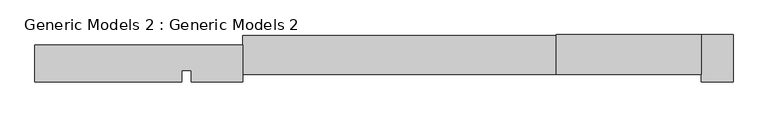
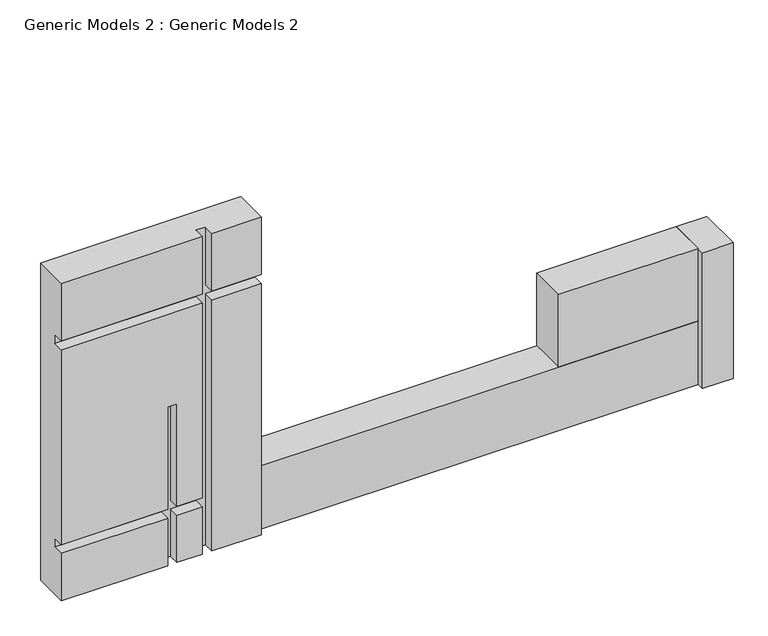
"""IFC4 building model written with IfcOpenShell, lengths in millimetres: proxy geometry, Generic Models 2 : Generic Models 2."""

from ifc_helpers import new_model, si_unit, frame, origin, place, context, project, spatial, polyline, outline, extrude, faceted_brep, source, transform, mapped, element, save


def generic_models_2_generic_models_2_1caf7409(model_context):
    return source(origin(), model_context, "Body", "SolidModel", [
        extrude(outline(polyline([(7416.0108478, -4009.874389), (7416.0108478, -3491.6545867), (9316.5582436, -3491.6545867), (9316.5582436, -4009.874389), (7416.0108478, -4009.874389)])), frame((0.0, 0.0, 4267.2), z_axis=(0.0, 0.0, 1.0), x_axis=(1.0, 0.0, 0.0)), (0.0, 0.0, 1.0), 1041.4),
        extrude(outline(polyline([(9733.554407, -4111.474389), (9316.5582436, -4111.474389), (9316.5582436, -3491.6545867), (9733.554407, -3491.6545867), (9733.554407, -4111.474389)])), frame((0.0, 0.0, 3352.8), z_axis=(0.0, 0.0, 1.0), x_axis=(1.0, 0.0, 0.0)), (0.0, 0.0, 1.0), 1955.8),
        extrude(outline(polyline([(9316.5582436, -4009.874389), (3313.273546, -4009.874389), (3313.273546, -3501.874389), (9316.5582436, -3501.874389), (9316.5582436, -4009.874389)])), frame((0.0, 0.0, 3352.8), z_axis=(0.0, 0.0, 1.0), x_axis=(1.0, 0.0, 0.0)), (0.0, 0.0, 1.0), 914.4),
        faceted_brep([(3313.273546, -4111.474389, 7924.8), (2638.6516969, -4111.474389, 7924.8), (2638.6516969, -4111.474389, 7095.4038204), (3313.273546, -4111.474389, 7095.4038204), (2511.6516969, -4111.474389, 7924.8), (589.554407, -4111.474389, 7924.8), (589.554407, -4111.474389, 7095.4038204), (2511.6516969, -4111.474389, 7095.4038204), (2638.6516969, -4111.474389, 3352.8), (3313.273546, -4111.474389, 3352.8), (3313.273546, -4111.474389, 6968.4038204), (2638.6516969, -4111.474389, 6968.4038204), (2511.6516969, -4111.474389, 6968.4038204), (589.554407, -4111.474389, 6968.4038204), (589.554407, -4111.474389, 4161.5389733), (2036.3810407, -4111.474389, 4161.5389733), (2036.3810407, -4111.474389, 5638.8), (2163.3810407, -4111.474389, 5638.8), (2163.3810407, -4111.474389, 4161.5389733), (2511.6516969, -4111.474389, 4161.5389733), (2511.6516969, -4111.474389, 3352.8), (2511.6516969, -4111.474389, 4034.5389733), (2163.3810407, -4111.474389, 4034.5389733), (2163.3810407, -4111.474389, 3352.8), (589.554407, -4111.474389, 4034.5389733), (589.554407, -4111.474389, 3352.8), (2036.3810407, -4111.474389, 3352.8), (2036.3810407, -4111.474389, 4034.5389733), (3313.273546, -3629.4798155, 7924.8), (3313.273546, -3629.4798155, 3352.8), (589.554407, -3629.4798155, 3352.8), (589.554407, -3629.4798155, 7924.8), (2511.6516969, -3959.074389, 7924.8), (2638.6516969, -3959.074389, 7924.8), (589.554407, -3959.074389, 4034.5389733), (589.554407, -3959.074389, 4161.5389733), (589.554407, -3959.074389, 6968.4038204), (589.554407, -3959.074389, 7095.4038204), (2638.6516969, -3959.074389, 3352.8), (2511.6516969, -3959.074389, 3352.8), (2163.3810407, -3959.074389, 3352.8), (2036.3810407, -3959.074389, 3352.8), (3313.273546, -3959.074389, 7095.4038204), (3313.273546, -3959.074389, 6968.4038204), (2511.6516969, -3959.074389, 7095.4038204), (2511.6516969, -3959.074389, 6968.4038204), (2511.6516969, -3959.074389, 4161.5389733), (2163.3810407, -3959.074389, 4161.5389733), (2163.3810407, -3959.074389, 5638.8), (2036.3810407, -3959.074389, 5638.8), (2036.3810407, -3959.074389, 4161.5389733), (2036.3810407, -3959.074389, 4034.5389733), (2163.3810407, -3959.074389, 4034.5389733), (2511.6516969, -3959.074389, 4034.5389733), (2638.6516969, -3959.074389, 6968.4038204), (2638.6516969, -3959.074389, 7095.4038204)], [[[0, 1, 2, 3]], [[4, 5, 6, 7]], [[8, 9, 10, 11]], [[12, 13, 14, 15, 16, 17, 18, 19]], [[20, 21, 22, 23]], [[24, 25, 26, 27]], [[28, 29, 30, 31]], [[28, 31, 5, 4, 32, 33, 1, 0]], [[31, 30, 25, 24, 34, 35, 14, 13, 36, 37, 6, 5]], [[30, 29, 9, 8, 38, 39, 20, 23, 40, 41, 26, 25]], [[29, 28, 0, 3, 42, 43, 10, 9]], [[33, 32, 44, 37, 36, 45, 46, 47, 48, 49, 50, 35, 34, 51, 41, 40, 52, 53, 39, 38, 54, 43, 42, 55]], [[1, 33, 55, 2]], [[38, 8, 11, 54]], [[32, 4, 7, 44]], [[20, 39, 53, 21]], [[45, 12, 19, 46]], [[37, 44, 7, 6]], [[55, 42, 3, 2]], [[45, 36, 13, 12]], [[43, 54, 11, 10]], [[14, 35, 50, 15]], [[46, 19, 18, 47]], [[34, 24, 27, 51]], [[21, 53, 52, 22]], [[41, 51, 27, 26]], [[49, 16, 15, 50]], [[49, 48, 17, 16]], [[52, 40, 23, 22]], [[17, 48, 47, 18]]]),
    ])


if __name__ == "__main__":
    model = new_model("IFC4")
    model_context = context("Model", 3, world=origin())
    ifc_project = project(units=[si_unit("LENGTHUNIT", "METRE", prefix="MILLI")], contexts=[model_context])
    site = spatial("IfcSite", under=ifc_project)
    building = spatial("IfcBuilding", under=site)
    placement = place(None, origin())
    generic_models_2_generic_models_2_shape = generic_models_2_generic_models_2_1caf7409(model_context)
    element("IfcBuildingElementProxy", 1, Name="Generic Models 2 : Generic Models 2", ObjectType="Generic Models 2 : Generic Models 2", at=placement, inside=building, context=model_context, shape_type="MappedRepresentation", body=[
        mapped(generic_models_2_generic_models_2_shape, transform((0.0, 0.0, 0.0), x_axis=(1.0, 0.0, 0.0), y_axis=(0.0, 1.0, 0.0), z_axis=(0.0, 0.0, 1.0))),
    ])
    save(model, "model.ifc")

# Revit data of these elements
# Element 1 (IfcBuildingElementProxy, "Generic Models 2 : Generic Models 2")
#   Materials on its faces: "Asphalt Shingle", "OLIVE GREY", "LIGHT GREY WHITE", "Wood Planks"
# Materials
#   "Asphalt Shingle": class "Generic", colour RGB 155 155 155, transparency 0, Description = "Asphalt roofing shingle", Cost = 0
#   "OLIVE GREY": class "Generic", colour RGB 120 120 120, transparency 0, Cost = 0
#   "LIGHT GREY WHITE": class "Generic", colour RGB 120 120 120, transparency 0, Cost = 0
#   "Wood Planks": class "Wood", colour RGB 193 160 115, transparency 0, Description = "Physical material.", Cost = 0
